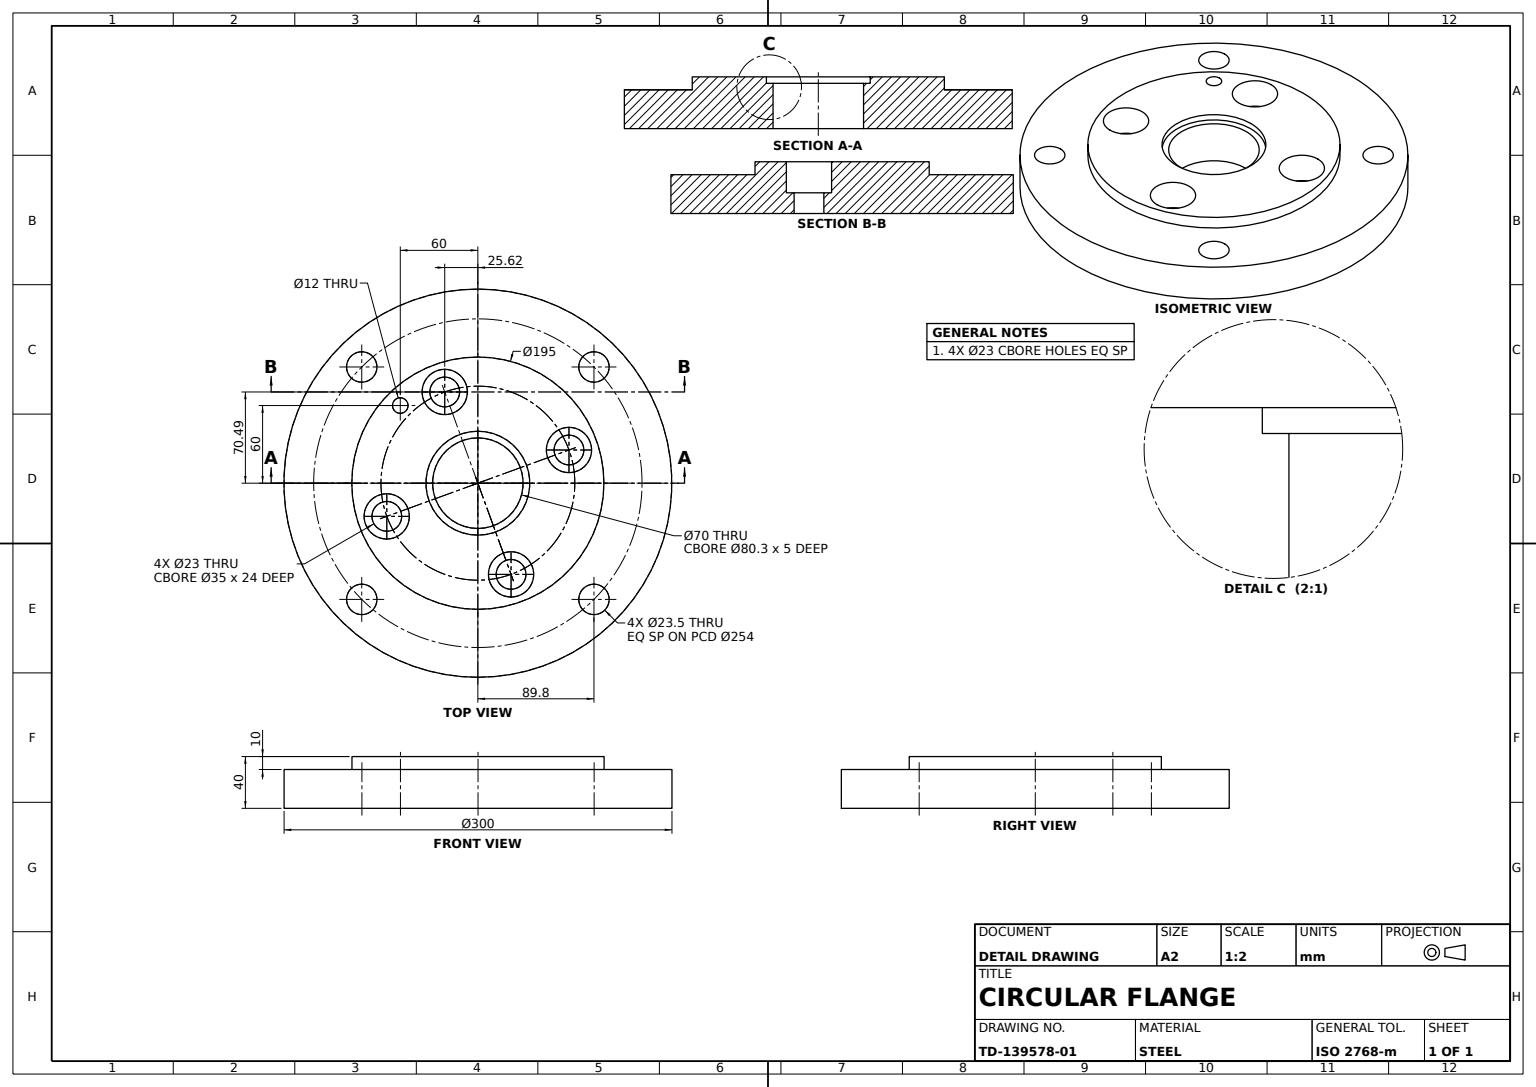
SolidWorks part; units mm, degrees
material "Plain Carbon Steel"
ref_plane "Front Plane" through (0, 0, 0) normal (0, 0, 1) x (1, 0, 0)
ref_plane "Top Plane" through (0, 0, 0) normal (0, 1, 0) x (1, 0, 0)
ref_plane "Right Plane" through (0, 0, 0) normal (1, 0, 0) x (0, 0, -1)
sketch "Flange Disc Sketch Ø300" plane through (0, 0, 0) normal (0, 1, 0) x (1, 0, 0)
  circle A0 centre (0, 0) radius 150
  dimension "D1" = 300
extrude "Flange Disc Ø300x40" add sketch "Flange Disc Sketch Ø300" against normal blind 40
sketch "Bore Sketch Ø70" plane through (0, 0, 0) normal (0, 1, 0) x (1, 0, 0)
  circle A0 centre (0, 0) radius 35
  dimension "D1" = 70
extrude "Bore Ø70 Through" cut sketch "Bore Sketch Ø70" against normal blind 40
sketch "Bore Recess Sketch Ø80.3" plane through (0, 0, 0) normal (0, 1, 0) x (1, 0, 0)
  circle A0 centre (0, 0) radius 35
  circle A1 centre (0, 0) radius 40.15
  dimension "D1" = 70
  dimension "D2" = 80.3
extrude "Bore Recess Ø80.3x5" cut sketch "Bore Recess Sketch Ø80.3" against normal blind 5
sketch "Raised Face Step Sketch" plane through (0, 0, 0) normal (0, 1, 0) x (1, 0, 0)
  circle A0 centre (0, 0) radius 97.5
  circle A1 centre (0, 0) radius 150
  dimension "D1" = 195
  dimension "D2" = 300
extrude "Raised Face Step Ø195x10" cut sketch "Raised Face Step Sketch" against normal blind 10
sketch "Outer Bolt Holes Sketch PCD254" plane through (0, -10, 0) normal (0, 1, 0) x (1, 0, 0)
  line L0 (-150, 0) -> (150, 0) construction
  line L1 (0, 150) -> (0, -150) construction
  line L2 (0, 0) -> (106.066, 106.066) construction
  circle A0 centre (0, 0) radius 127 construction
  circle A1 centre (0, 0) radius 150 construction
  circle A2 centre (89.8026, 89.8026) radius 11.75
  circle A3 centre (-89.8026, 89.8026) radius 11.75
  circle A4 centre (-89.8026, -89.8026) radius 11.75
  circle A5 centre (89.8026, -89.8026) radius 11.75
  dimension "D1" = 254
  dimension "D2" = 23.5
  dimension "D3" = 45
extrude "Outer Bolt Holes PCD254" cut sketch "Outer Bolt Holes Sketch PCD254" against normal through all
sketch "Inner Holes Sketch" plane through (0, 0, 0) normal (0, 1, 0) x (1, 0, 0)
  line L0 (0, 0) -> (140.9539, 51.303) construction
  line L1 (0, 0) -> (150, 0) construction
  line L2 (0, 150) -> (0, -150) construction
  line L3 (-150, 0) -> (0, 0) construction
  line L4 (0, 0) -> (-51.303, 140.9539) construction
  line L5 (0, 0) -> (-140.9539, -51.303) construction
  line L6 (0, 0) -> (51.303, -140.9539) construction
  circle A0 centre (0, 0) radius 150 construction
  circle A2 centre (-70.4769, -25.6515) radius 17.5
  circle A11 centre (0, 0) radius 75
  circle A12 centre (70.4769, 25.6515) radius 17.5
  circle A13 centre (-25.6168, 70.4896) radius 17.5
  circle A14 centre (25.6863, -70.4643) radius 17.5
  dimension "D1" = 35
  dimension "D2" = 35
  dimension "D7" = 70.4896
  dimension "D3" = 20
  dimension "D4" = 20
  dimension "D5" = 20
  dimension "D6" = 20
extrude "Inner Holes Cut 24 Deep" cut sketch "Inner Holes Sketch" against normal blind 24 contours A11 A13 | A11 A13 | A11 A12 | A11 A12 | A11 A2 | A2 A11 | A14 A11 | A14 A11
sketch "Inner Hole Secondary Sketch" plane through (0, 0, 0) normal (0, 1, 0) x (1, 0, 0)
  line L0 (70.4769, 25.6515) -> (-70.4769, -25.6515) construction
  line L1 (-25.6168, 70.4896) -> (25.6863, -70.4643) construction
  circle A0 centre (70.4769, 25.6515) radius 11.5
  circle A1 centre (-70.4075, -25.6262) radius 11.5
  circle A2 centre (-25.6168, 70.4896) radius 11.5
  circle A3 centre (25.6863, -70.4643) radius 11.5
  dimension "D1" = 23
  dimension "D2" = 23
extrude "Inner Hole Secondary Cut" cut sketch "Inner Hole Secondary Sketch" against normal through all
sketch "Small Hole Sketch Ø12" plane through (0, 0, 0) normal (0, 1, 0) x (1, 0, 0)
  line L0 (0, 0) -> (-60, 0) construction
  line L1 (-60, 0) -> (-60, 60) construction
  circle A0 centre (-60, 60) radius 6
  dimension "D1" = 12
  dimension "D2" = 60
  dimension "D3" = 60
extrude "Small Hole Ø12" cut sketch "Small Hole Sketch Ø12" against normal through all
